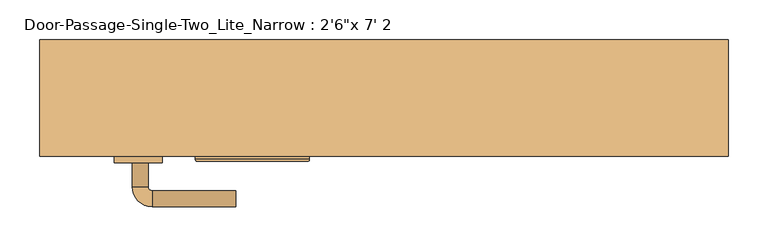
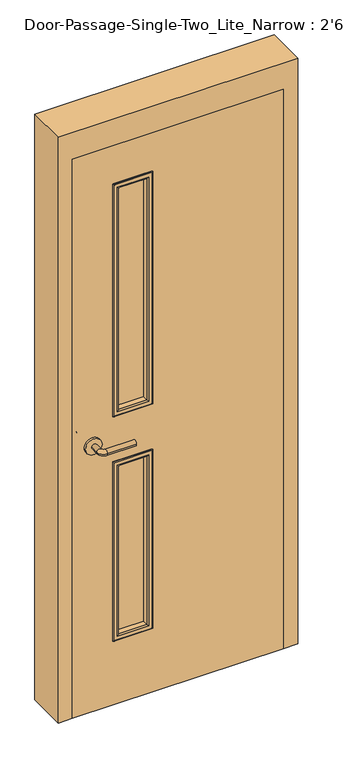
"""IFC4 building model written with IfcOpenShell, lengths in millimetres: door geometry."""

from ifc_helpers import new_model, si_unit, point, frame, frame_2d, origin, place, context, project, spatial, polyline, circle_curve, ellipse_curve, trimmed, segment, composite_curve, outline, extrude, faceted_brep, source, transform, mapped, element, save
from ifc_brep_helpers import plane_surface, cylinder_surface, revolved_surface, advanced_brep


def door_bcd1f9a3(model_context):
    return source(origin(), model_context, "Body", "SolidModel", [
        advanced_brep(
        [(-315.990625, 14.35, 1016.0), (-295.990625, 14.35, 1016.0), (-315.990625, 44.35, 1016.0), (-295.990625, 44.35, 1016.0), (-290.990625, 49.35, 1016.0), (-290.990625, 69.35, 1016.0), (-185.990625, 69.35, 1016.0), (-185.990625, 49.35, 1016.0)],
        [
            (0, 1, circle_curve(frame((-305.990625, 14.35, 1016.0), z_axis=(0.0, -1.0, 0.0), x_axis=(1.0, 0.0, 0.0)), 10.0)),
            (1, 0, circle_curve(frame((-305.990625, 14.35, 1016.0), z_axis=(0.0, -1.0, 0.0), x_axis=(1.0, 0.0, 0.0)), 10.0)),
            (0, 2),
            (2, 3, circle_curve(frame((-305.990625, 44.35, 1016.0), z_axis=(0.0, -1.0, 0.0), x_axis=(1.0, 0.0, 0.0)), 10.0)),
            (3, 1),
            (3, 2, circle_curve(frame((-305.990625, 44.35, 1016.0), z_axis=(0.0, -1.0, 0.0), x_axis=(1.0, 0.0, 0.0)), 10.0)),
            (4, 3, circle_curve(frame((-290.990625, 44.35, 1016.0), z_axis=(0.0, 0.0, 1.0), x_axis=(-1.0, 0.0, 0.0)), 5.0)),
            (2, 5, circle_curve(frame((-290.990625, 44.35, 1016.0), z_axis=(0.0, 0.0, -1.0), x_axis=(-1.0, 0.0, 0.0)), 25.0)),
            (5, 4, circle_curve(frame((-290.990625, 59.35, 1016.0), z_axis=(-1.0, 0.0, 0.0), x_axis=(0.0, -1.0, 0.0)), 10.0)),
            (4, 5, circle_curve(frame((-290.990625, 59.35, 1016.0), z_axis=(-1.0, 0.0, 0.0), x_axis=(0.0, -1.0, 0.0)), 10.0)),
            (6, 7, circle_curve(frame((-185.990625, 59.35, 1016.0), z_axis=(1.0, 0.0, 0.0), x_axis=(0.0, -1.0, 0.0)), 10.0)),
            (7, 6, circle_curve(frame((-185.990625, 59.35, 1016.0), z_axis=(1.0, 0.0, 0.0), x_axis=(0.0, -1.0, 0.0)), 10.0)),
            (5, 6),
            (7, 4),
        ],
        [
            plane_surface(frame((-305.990625, 14.35, 1016.0), z_axis=(0.0, -1.0, 0.0), x_axis=(0.0, 0.0, 1.0))),
            cylinder_surface(frame((-305.990625, 14.35, 1016.0), z_axis=(0.0, -1.0, 0.0), x_axis=(1.0, 0.0, 0.0)), 10.0),
            revolved_surface(trimmed(ellipse_curve(frame((-305.990625, 44.35, 1016.0), z_axis=(0.0, -1.0, 0.0), x_axis=(1.0, 0.0, 0.0)), 10.0, 10.0), [point((-315.990625, 44.35, 1016.0))], [point((-295.990625, 44.35, 1016.0))], True, "CARTESIAN"), (-290.990625, 44.35, 1016.0), (0.0, 0.0, -1.0)),
            revolved_surface(trimmed(ellipse_curve(frame((-305.990625, 44.35, 1016.0), z_axis=(0.0, -1.0, 0.0), x_axis=(1.0, 0.0, 0.0)), 10.0, 10.0), [point((-295.990625, 44.35, 1016.0))], [point((-315.990625, 44.35, 1016.0))], True, "CARTESIAN"), (-290.990625, 44.35, 1016.0), (0.0, 0.0, -1.0)),
            plane_surface(frame((-185.990625, 59.35, 1016.0), z_axis=(1.0, 0.0, 0.0), x_axis=(0.0, 0.0, 1.0))),
            cylinder_surface(frame((-290.990625, 59.35, 1016.0), z_axis=(-1.0, 0.0, 0.0), x_axis=(0.0, -1.0, 0.0)), 10.0),
        ],
        [
            (0, [[1, 2]]),
            (1, [[-1, 3, 4, 5]]),
            (1, [[-2, -5, 6, -3]]),
            (2, [[7, -4, 8, 9]]),
            (3, [[-8, -6, -7, 10]]),
            (4, [[11, 12]]),
            (5, [[-9, 13, -12, 14]]),
            (5, [[-10, -14, -11, -13]]),
        ],
    ),
        extrude(outline(composite_curve([segment(trimmed(circle_curve(frame_2d((1016.0, -308.490625)), 30.0), [point((1016.0, -338.490625))], [point((1016.0, -278.490625))], False, "CARTESIAN"), True, "CONTINUOUS"), segment(trimmed(circle_curve(frame_2d((1016.0, -308.490625)), 30.0), [point((1016.0, -278.490625))], [point((1016.0, -338.490625))], False, "CARTESIAN"), True, "CONTINUOUS")], self_intersect=False)), frame((0.0, 6.35, 0.0), z_axis=(0.0, 1.0, 0.0), x_axis=(0.0, 0.0, 1.0)), (0.0, 0.0, 1.0), 8.0),
        advanced_brep(
        [(-315.990625, -46.1, 1016.0), (-295.990625, -46.1, 1016.0), (-295.990625, -76.1, 1016.0), (-315.990625, -76.1, 1016.0), (-290.990625, -81.1, 1016.0), (-290.990625, -101.1, 1016.0), (-185.990625, -101.1, 1016.0), (-185.990625, -81.1, 1016.0)],
        [
            (0, 1, circle_curve(frame((-305.990625, -46.1, 1016.0), z_axis=(0.0, 1.0, 0.0), x_axis=(1.0, 0.0, 0.0)), 10.0)),
            (1, 0, circle_curve(frame((-305.990625, -46.1, 1016.0), z_axis=(0.0, 1.0, 0.0), x_axis=(1.0, 0.0, 0.0)), 10.0)),
            (1, 2),
            (2, 3, circle_curve(frame((-305.990625, -76.1, 1016.0), z_axis=(0.0, 1.0, 0.0), x_axis=(1.0, 0.0, 0.0)), 10.0)),
            (3, 0),
            (3, 2, circle_curve(frame((-305.990625, -76.1, 1016.0), z_axis=(0.0, 1.0, 0.0), x_axis=(1.0, 0.0, 0.0)), 10.0)),
            (4, 5, circle_curve(frame((-290.990625, -91.1, 1016.0), z_axis=(-1.0, 0.0, 0.0), x_axis=(0.0, 1.0, 0.0)), 10.0)),
            (5, 3, circle_curve(frame((-290.990625, -76.1, 1016.0), z_axis=(0.0, 0.0, -1.0), x_axis=(-1.0, 0.0, 0.0)), 25.0)),
            (2, 4, circle_curve(frame((-290.990625, -76.1, 1016.0), z_axis=(0.0, 0.0, 1.0), x_axis=(-1.0, 0.0, 0.0)), 5.0)),
            (5, 4, circle_curve(frame((-290.990625, -91.1, 1016.0), z_axis=(-1.0, 0.0, 0.0), x_axis=(0.0, 1.0, 0.0)), 10.0)),
            (6, 7, circle_curve(frame((-185.990625, -91.1, 1016.0), z_axis=(1.0, 0.0, 0.0), x_axis=(0.0, 1.0, 0.0)), 10.0)),
            (7, 6, circle_curve(frame((-185.990625, -91.1, 1016.0), z_axis=(1.0, 0.0, 0.0), x_axis=(0.0, 1.0, 0.0)), 10.0)),
            (4, 7),
            (6, 5),
        ],
        [
            plane_surface(frame((-305.990625, -46.1, 1016.0), z_axis=(0.0, 1.0, 0.0), x_axis=(0.0, 0.0, 1.0))),
            cylinder_surface(frame((-305.990625, -46.1, 1016.0), z_axis=(0.0, 1.0, 0.0), x_axis=(1.0, 0.0, 0.0)), 10.0),
            revolved_surface(trimmed(ellipse_curve(frame((-305.990625, -76.1, 1016.0), z_axis=(0.0, -1.0, 0.0), x_axis=(1.0, 0.0, 0.0)), 10.0, 10.0), [point((-315.990625, -76.1, 1016.0))], [point((-295.990625, -76.1, 1016.0))], True, "CARTESIAN"), (-290.990625, -76.1, 1016.0), (0.0, 0.0, -1.0)),
            revolved_surface(trimmed(ellipse_curve(frame((-305.990625, -76.1, 1016.0), z_axis=(0.0, -1.0, 0.0), x_axis=(1.0, 0.0, 0.0)), 10.0, 10.0), [point((-295.990625, -76.1, 1016.0))], [point((-315.990625, -76.1, 1016.0))], True, "CARTESIAN"), (-290.990625, -76.1, 1016.0), (0.0, 0.0, -1.0)),
            plane_surface(frame((-185.990625, -91.1, 1016.0), z_axis=(1.0, 0.0, 0.0), x_axis=(0.0, 0.0, 1.0))),
            cylinder_surface(frame((-290.990625, -91.1, 1016.0), z_axis=(-1.0, 0.0, 0.0), x_axis=(0.0, 1.0, 0.0)), 10.0),
        ],
        [
            (0, [[1, 2]]),
            (1, [[3, 4, 5, -2]]),
            (1, [[-5, 6, -3, -1]]),
            (2, [[7, 8, -4, 9]]),
            (3, [[10, -9, -6, -8]]),
            (4, [[11, 12]]),
            (5, [[13, -11, 14, -7]]),
            (5, [[-14, -12, -13, -10]]),
        ],
    ),
        extrude(outline(composite_curve([segment(trimmed(circle_curve(frame_2d((1016.0, -308.490625)), 30.0), [point((1016.0, -338.490625))], [point((1016.0, -278.490625))], False, "CARTESIAN"), True, "CONTINUOUS"), segment(trimmed(circle_curve(frame_2d((1016.0, -308.490625)), 30.0), [point((1016.0, -278.490625))], [point((1016.0, -338.490625))], False, "CARTESIAN"), True, "CONTINUOUS")], self_intersect=False)), frame((0.0, -46.1, 0.0), z_axis=(0.0, 1.0, 0.0), x_axis=(0.0, 0.0, 1.0)), (0.0, 0.0, 1.0), 8.0),
        extrude(outline(polyline([(2133.6, -381.0), (0.0, -381.0), (0.0, 381.0), (2133.6, 381.0), (2133.6, -381.0)]), holes=[polyline([(1981.2, -228.6), (1981.2, -101.6), (1111.25, -101.6), (1111.25, -228.6), (1981.2, -228.6)]), polyline([(920.75, -228.6), (920.75, -101.6), (254.0, -101.6), (254.0, -228.6), (920.75, -228.6)])]), frame((0.0, -38.1, 0.0), z_axis=(0.0, 1.0, 0.0), x_axis=(0.0, 0.0, 1.0)), (0.0, 0.0, 1.0), 44.45),
        faceted_brep([(381.0, 11.1125, 0.0), (365.125, 11.1125, 0.0), (365.125, 58.7375, 0.0), (381.0, 58.7375, 0.0), (381.0, 107.95, 0.0), (431.8, 107.95, 0.0), (431.8, -38.1, 0.0), (381.0, -38.1, 0.0), (381.0, -38.1, 2133.6), (381.0, 11.1125, 2133.6), (431.8, -38.1, 2235.2), (-431.8, -38.1, 2235.2), (-431.8, -38.1, 0.0), (-381.0, -38.1, 0.0), (-381.0, -38.1, 2133.6), (431.8, 107.95, 2235.2), (381.0, 107.95, 2133.6), (-381.0, 107.95, 2133.6), (-381.0, 107.95, 0.0), (-431.8, 107.95, 0.0), (-431.8, 107.95, 2235.2), (381.0, 58.7375, 2133.6), (365.125, 58.7375, 2117.725), (-365.125, 58.7375, 2117.725), (-365.125, 58.7375, 0.0), (-381.0, 58.7375, 0.0), (-381.0, 58.7375, 2133.6), (365.125, 11.1125, 2117.725), (-381.0, 11.1125, 2133.6), (-381.0, 11.1125, 0.0), (-365.125, 11.1125, 0.0), (-365.125, 11.1125, 2117.725)], [[[0, 1, 2, 3, 4, 5, 6, 7]], [[7, 8, 9, 0]], [[6, 10, 11, 12, 13, 14, 8, 7]], [[5, 15, 10, 6]], [[4, 16, 17, 18, 19, 20, 15, 5]], [[3, 21, 16, 4]], [[2, 22, 23, 24, 25, 26, 21, 3]], [[1, 27, 22, 2]], [[0, 9, 28, 29, 30, 31, 27, 1]], [[8, 14, 28, 9]], [[16, 21, 26, 17]], [[22, 27, 31, 23]], [[12, 19, 18, 25, 24, 30, 29, 13]], [[13, 29, 28, 14]], [[11, 20, 19, 12]], [[17, 26, 25, 18]], [[23, 31, 30, 24]], [[15, 20, 11, 10]]]),
        extrude(outline(polyline([(-101.6, -12.7), (-101.6, -19.05), (-228.6, -19.05), (-228.6, -12.7), (-101.6, -12.7)])), frame((0.0, 0.0, 1111.25), z_axis=(0.0, 0.0, 1.0), x_axis=(1.0, 0.0, 0.0)), (0.0, 0.0, 1.0), 869.95),
        extrude(outline(polyline([(-101.6, -12.7), (-101.6, -19.05), (-228.6, -19.05), (-228.6, -12.7), (-101.6, -12.7)])), frame((0.0, 0.0, 254.0), z_axis=(0.0, 0.0, 1.0), x_axis=(1.0, 0.0, 0.0)), (0.0, 0.0, 1.0), 666.75),
        advanced_brep(
        [(-228.6, -19.05, 1981.2), (-228.6, -19.05, 1111.25), (-228.6, -38.1, 1111.25), (-228.6, -38.1, 1981.2), (-216.6, -39.1, 1969.2), (-216.6, -39.1, 1123.25), (-216.6, -19.05, 1123.25), (-216.6, -19.05, 1969.2), (-221.6, -44.1, 1974.2), (-221.6, -44.1, 1118.25), (-236.6, -42.1, 1989.2), (-236.6, -42.1, 1103.25), (-234.6, -44.1, 1105.25), (-234.6, -44.1, 1987.2), (-236.6, -38.1, 1989.2), (-236.6, -38.1, 1103.25), (-101.6, -19.05, 1111.25), (-101.6, -38.1, 1111.25), (-113.6, -39.1, 1123.25), (-113.6, -19.05, 1123.25), (-108.6, -44.1, 1118.25), (-93.6, -42.1, 1103.25), (-95.6, -44.1, 1105.25), (-93.6, -38.1, 1103.25), (-101.6, -19.05, 1981.2), (-101.6, -38.1, 1981.2), (-113.6, -39.1, 1969.2), (-113.6, -19.05, 1969.2), (-108.6, -44.1, 1974.2), (-93.6, -42.1, 1989.2), (-95.6, -44.1, 1987.2), (-93.6, -38.1, 1989.2)],
        [
            (0, 1),
            (1, 2),
            (2, 3),
            (3, 0),
            (4, 5),
            (5, 6),
            (6, 7),
            (7, 4),
            (8, 9),
            (9, 5, ellipse_curve(frame((-221.6, -39.1, 1118.25), z_axis=(-0.7071067811865475, 0.0, 0.7071067811865475), x_axis=(0.7071067811865474, 0.0, 0.7071067811865476)), 7.0710678, 5.0)),
            (4, 8, ellipse_curve(frame((-221.6, -39.1, 1974.2), z_axis=(-0.7071067811865475, 0.0, -0.7071067811865475), x_axis=(-0.7071067811865474, 0.0, 0.7071067811865476)), 7.0710678, 5.0)),
            (10, 11),
            (11, 12, ellipse_curve(frame((-234.6, -42.1, 1105.25), z_axis=(-0.7071067811865475, 0.0, 0.7071067811865475), x_axis=(0.7071067811865474, 0.0, 0.7071067811865476)), 2.8284271, 2.0)),
            (12, 13),
            (13, 10, ellipse_curve(frame((-234.6, -42.1, 1987.2), z_axis=(-0.7071067811865475, 0.0, -0.7071067811865475), x_axis=(-0.7071067811865474, 0.0, 0.7071067811865476)), 2.8284271, 2.0)),
            (14, 15),
            (15, 11),
            (10, 14),
            (1, 16),
            (16, 17),
            (17, 2),
            (5, 18),
            (18, 19),
            (19, 6),
            (9, 20),
            (20, 18, ellipse_curve(frame((-108.6, -39.1, 1118.25), z_axis=(-0.7071067811865475, 0.0, -0.7071067811865475), x_axis=(-0.7071067811865476, 0.0, 0.7071067811865474)), 7.0710678, 5.0)),
            (11, 21),
            (21, 22, ellipse_curve(frame((-95.6, -42.1, 1105.25), z_axis=(-0.7071067811865475, 0.0, -0.7071067811865475), x_axis=(-0.7071067811865476, 0.0, 0.7071067811865474)), 2.8284271, 2.0)),
            (22, 12),
            (15, 23),
            (23, 21),
            (16, 24),
            (24, 25),
            (25, 17),
            (18, 26),
            (26, 27),
            (27, 19),
            (20, 28),
            (28, 26, ellipse_curve(frame((-108.6, -39.1, 1974.2), z_axis=(0.7071067811865475, 0.0, -0.7071067811865475), x_axis=(-0.7071067811865474, 0.0, -0.7071067811865476)), 7.0710678, 5.0)),
            (21, 29),
            (29, 30, ellipse_curve(frame((-95.6, -42.1, 1987.2), z_axis=(0.7071067811865475, 0.0, -0.7071067811865475), x_axis=(-0.7071067811865474, 0.0, -0.7071067811865476)), 2.8284271, 2.0)),
            (30, 22),
            (23, 31),
            (31, 29),
            (14, 31),
            (25, 3),
            (24, 0),
            (27, 7),
            (26, 4),
            (28, 8),
            (30, 13),
            (29, 10),
        ],
        [
            plane_surface(frame((-228.6, -38.1, 1981.2), z_axis=(-1.0, 0.0, 0.0), x_axis=(0.0, 0.0, -1.0))),
            plane_surface(frame((-216.6, -19.05, 1969.2), z_axis=(1.0, 0.0, 0.0), x_axis=(0.0, 0.0, -1.0))),
            cylinder_surface(frame((-221.6, -39.1, 1981.2), z_axis=(0.0, 0.0, 1.0), x_axis=(-1.0, 0.0, 0.0)), 5.0),
            cylinder_surface(frame((-234.6, -42.1, 1981.2), z_axis=(0.0, 0.0, 1.0), x_axis=(-1.0, 0.0, 0.0)), 2.0),
            plane_surface(frame((-236.6, -42.1, 1989.2), z_axis=(-1.0, 0.0, 0.0), x_axis=(0.0, 0.0, -1.0))),
            plane_surface(frame((-228.6, -38.1, 1111.25), z_axis=(0.0, 0.0, -1.0), x_axis=(1.0, 0.0, 0.0))),
            plane_surface(frame((-216.6, -19.05, 1123.25), z_axis=(0.0, 0.0, 1.0), x_axis=(1.0, 0.0, 0.0))),
            cylinder_surface(frame((-228.6, -39.1, 1118.25), z_axis=(-1.0, 0.0, 0.0), x_axis=(0.0, 0.0, -1.0)), 5.0),
            cylinder_surface(frame((-228.6, -42.1, 1105.25), z_axis=(-1.0, 0.0, 0.0), x_axis=(0.0, 0.0, -1.0)), 2.0),
            plane_surface(frame((-236.6, -42.1, 1103.25), z_axis=(0.0, 0.0, -1.0), x_axis=(1.0, 0.0, 0.0))),
            plane_surface(frame((-101.6, -38.1, 1111.25), z_axis=(1.0, 0.0, 0.0), x_axis=(0.0, 0.0, 1.0))),
            plane_surface(frame((-113.6, -19.05, 1123.25), z_axis=(-1.0, 0.0, 0.0), x_axis=(0.0, 0.0, 1.0))),
            cylinder_surface(frame((-108.6, -39.1, 1111.25), z_axis=(0.0, 0.0, -1.0), x_axis=(1.0, 0.0, 0.0)), 5.0),
            cylinder_surface(frame((-95.6, -42.1, 1111.25), z_axis=(0.0, 0.0, -1.0), x_axis=(1.0, 0.0, 0.0)), 2.0),
            plane_surface(frame((-93.6, -42.1, 1103.25), z_axis=(1.0, 0.0, 0.0), x_axis=(0.0, 0.0, 1.0))),
            plane_surface(frame((-93.6, -38.1, 1989.2), z_axis=(0.0, 1.0, 0.0), x_axis=(-1.0, 0.0, 0.0))),
            plane_surface(frame((-101.6, -38.1, 1981.2), z_axis=(0.0, 0.0, 1.0), x_axis=(-1.0, 0.0, 0.0))),
            plane_surface(frame((-101.6, -19.05, 1981.2), z_axis=(0.0, 1.0, 0.0), x_axis=(-1.0, 0.0, 0.0))),
            plane_surface(frame((-113.6, -19.05, 1969.2), z_axis=(0.0, 0.0, -1.0), x_axis=(-1.0, 0.0, 0.0))),
            cylinder_surface(frame((-101.6, -39.1, 1974.2), z_axis=(1.0, 0.0, 0.0), x_axis=(0.0, 0.0, 1.0)), 5.0),
            plane_surface(frame((-108.6, -44.1, 1974.2), z_axis=(0.0, -1.0, 0.0), x_axis=(-1.0, 0.0, 0.0))),
            cylinder_surface(frame((-101.6, -42.1, 1987.2), z_axis=(1.0, 0.0, 0.0), x_axis=(0.0, 0.0, 1.0)), 2.0),
            plane_surface(frame((-93.6, -42.1, 1989.2), z_axis=(0.0, 0.0, 1.0), x_axis=(-1.0, 0.0, 0.0))),
        ],
        [
            (0, [[1, 2, 3, 4]]),
            (1, [[5, 6, 7, 8]]),
            (2, [[9, 10, -5, 11]]),
            (3, [[12, 13, 14, 15]]),
            (4, [[16, 17, -12, 18]]),
            (5, [[19, 20, 21, -2]]),
            (6, [[22, 23, 24, -6]]),
            (7, [[25, 26, -22, -10]]),
            (8, [[27, 28, 29, -13]]),
            (9, [[30, 31, -27, -17]]),
            (10, [[32, 33, 34, -20]]),
            (11, [[35, 36, 37, -23]]),
            (12, [[38, 39, -35, -26]]),
            (13, [[40, 41, 42, -28]]),
            (14, [[43, 44, -40, -31]]),
            (15, [[-16, 45, -43, -30], [-3, -21, -34, 46]]),
            (16, [[47, -4, -46, -33]]),
            (17, [[-1, -47, -32, -19], [-7, -24, -37, 48]]),
            (18, [[49, -8, -48, -36]]),
            (19, [[50, -11, -49, -39]]),
            (20, [[-14, -29, -42, 51], [-9, -50, -38, -25]]),
            (21, [[52, -15, -51, -41]]),
            (22, [[-45, -18, -52, -44]]),
        ],
    ),
        advanced_brep(
        [(-228.6, -12.7, 1111.25), (-228.6, -12.7, 1981.2), (-228.6, 6.35, 1981.2), (-228.6, 6.35, 1111.25), (-216.6, 7.35, 1123.25), (-216.6, 7.35, 1969.2), (-216.6, -12.7, 1969.2), (-216.6, -12.7, 1123.25), (-221.6, 12.35, 1118.25), (-221.6, 12.35, 1974.2), (-236.6, 10.35, 1103.25), (-236.6, 10.35, 1989.2), (-234.6, 12.35, 1987.2), (-234.6, 12.35, 1105.25), (-236.6, 6.35, 1103.25), (-236.6, 6.35, 1989.2), (-101.6, -12.7, 1981.2), (-101.6, 6.35, 1981.2), (-113.6, 7.35, 1969.2), (-113.6, -12.7, 1969.2), (-108.6, 12.35, 1974.2), (-93.6, 10.35, 1989.2), (-95.6, 12.35, 1987.2), (-93.6, 6.35, 1989.2), (-101.6, -12.7, 1111.25), (-101.6, 6.35, 1111.25), (-113.6, 7.35, 1123.25), (-113.6, -12.7, 1123.25), (-108.6, 12.35, 1118.25), (-93.6, 10.35, 1103.25), (-95.6, 12.35, 1105.25), (-93.6, 6.35, 1103.25)],
        [
            (0, 1),
            (1, 2),
            (2, 3),
            (3, 0),
            (4, 5),
            (5, 6),
            (6, 7),
            (7, 4),
            (8, 9),
            (9, 5, ellipse_curve(frame((-221.6, 7.35, 1974.2), z_axis=(-0.7071067811865475, 0.0, -0.7071067811865475), x_axis=(0.7071067811865474, 0.0, -0.7071067811865476)), 7.0710678, 5.0)),
            (4, 8, ellipse_curve(frame((-221.6, 7.35, 1118.25), z_axis=(-0.7071067811865475, 0.0, 0.7071067811865475), x_axis=(-0.7071067811865474, 0.0, -0.7071067811865476)), 7.0710678, 5.0)),
            (10, 11),
            (11, 12, ellipse_curve(frame((-234.6, 10.35, 1987.2), z_axis=(-0.7071067811865475, 0.0, -0.7071067811865475), x_axis=(0.7071067811865474, 0.0, -0.7071067811865476)), 2.8284271, 2.0)),
            (12, 13),
            (13, 10, ellipse_curve(frame((-234.6, 10.35, 1105.25), z_axis=(-0.7071067811865475, 0.0, 0.7071067811865475), x_axis=(-0.7071067811865474, 0.0, -0.7071067811865476)), 2.8284271, 2.0)),
            (14, 15),
            (15, 11),
            (10, 14),
            (1, 16),
            (16, 17),
            (17, 2),
            (5, 18),
            (18, 19),
            (19, 6),
            (9, 20),
            (20, 18, ellipse_curve(frame((-108.6, 7.35, 1974.2), z_axis=(-0.7071067811865475, 0.0, 0.7071067811865475), x_axis=(-0.7071067811865476, 0.0, -0.7071067811865474)), 7.0710678, 5.0)),
            (11, 21),
            (21, 22, ellipse_curve(frame((-95.6, 10.35, 1987.2), z_axis=(-0.7071067811865475, 0.0, 0.7071067811865475), x_axis=(-0.7071067811865476, 0.0, -0.7071067811865474)), 2.8284271, 2.0)),
            (22, 12),
            (15, 23),
            (23, 21),
            (16, 24),
            (24, 25),
            (25, 17),
            (18, 26),
            (26, 27),
            (27, 19),
            (20, 28),
            (28, 26, ellipse_curve(frame((-108.6, 7.35, 1118.25), z_axis=(0.7071067811865475, 0.0, 0.7071067811865475), x_axis=(-0.7071067811865474, 0.0, 0.7071067811865476)), 7.0710678, 5.0)),
            (21, 29),
            (29, 30, ellipse_curve(frame((-95.6, 10.35, 1105.25), z_axis=(0.7071067811865475, 0.0, 0.7071067811865475), x_axis=(-0.7071067811865474, 0.0, 0.7071067811865476)), 2.8284271, 2.0)),
            (30, 22),
            (23, 31),
            (31, 29),
            (14, 31),
            (25, 3),
            (24, 0),
            (27, 7),
            (26, 4),
            (28, 8),
            (30, 13),
            (29, 10),
        ],
        [
            plane_surface(frame((-228.6, 6.35, 1111.25), z_axis=(-1.0, 0.0, 0.0), x_axis=(0.0, 0.0, 1.0))),
            plane_surface(frame((-216.6, -12.7, 1123.25), z_axis=(1.0, 0.0, 0.0), x_axis=(0.0, 0.0, 1.0))),
            cylinder_surface(frame((-221.6, 7.35, 1111.25), z_axis=(0.0, 0.0, -1.0), x_axis=(-1.0, 0.0, 0.0)), 5.0),
            cylinder_surface(frame((-234.6, 10.35, 1111.25), z_axis=(0.0, 0.0, -1.0), x_axis=(-1.0, 0.0, 0.0)), 2.0),
            plane_surface(frame((-236.6, 10.35, 1103.25), z_axis=(-1.0, 0.0, 0.0), x_axis=(0.0, 0.0, 1.0))),
            plane_surface(frame((-228.6, 6.35, 1981.2), z_axis=(0.0, 0.0, 1.0), x_axis=(1.0, 0.0, 0.0))),
            plane_surface(frame((-216.6, -12.7, 1969.2), z_axis=(0.0, 0.0, -1.0), x_axis=(1.0, 0.0, 0.0))),
            cylinder_surface(frame((-228.6, 7.35, 1974.2), z_axis=(-1.0, 0.0, 0.0), x_axis=(0.0, 0.0, 1.0)), 5.0),
            cylinder_surface(frame((-228.6, 10.35, 1987.2), z_axis=(-1.0, 0.0, 0.0), x_axis=(0.0, 0.0, 1.0)), 2.0),
            plane_surface(frame((-236.6, 10.35, 1989.2), z_axis=(0.0, 0.0, 1.0), x_axis=(1.0, 0.0, 0.0))),
            plane_surface(frame((-101.6, 6.35, 1981.2), z_axis=(1.0, 0.0, 0.0), x_axis=(0.0, 0.0, -1.0))),
            plane_surface(frame((-113.6, -12.7, 1969.2), z_axis=(-1.0, 0.0, 0.0), x_axis=(0.0, 0.0, -1.0))),
            cylinder_surface(frame((-108.6, 7.35, 1981.2), z_axis=(0.0, 0.0, 1.0), x_axis=(1.0, 0.0, 0.0)), 5.0),
            cylinder_surface(frame((-95.6, 10.35, 1981.2), z_axis=(0.0, 0.0, 1.0), x_axis=(1.0, 0.0, 0.0)), 2.0),
            plane_surface(frame((-93.6, 10.35, 1989.2), z_axis=(1.0, 0.0, 0.0), x_axis=(0.0, 0.0, -1.0))),
            plane_surface(frame((-93.6, 6.35, 1103.25), z_axis=(0.0, -1.0, 0.0), x_axis=(-1.0, 0.0, 0.0))),
            plane_surface(frame((-101.6, 6.35, 1111.25), z_axis=(0.0, 0.0, -1.0), x_axis=(-1.0, 0.0, 0.0))),
            plane_surface(frame((-101.6, -12.7, 1111.25), z_axis=(0.0, -1.0, 0.0), x_axis=(-1.0, 0.0, 0.0))),
            plane_surface(frame((-113.6, -12.7, 1123.25), z_axis=(0.0, 0.0, 1.0), x_axis=(-1.0, 0.0, 0.0))),
            cylinder_surface(frame((-101.6, 7.35, 1118.25), z_axis=(1.0, 0.0, 0.0), x_axis=(0.0, 0.0, -1.0)), 5.0),
            plane_surface(frame((-108.6, 12.35, 1118.25), z_axis=(0.0, 1.0, 0.0), x_axis=(-1.0, 0.0, 0.0))),
            cylinder_surface(frame((-101.6, 10.35, 1105.25), z_axis=(1.0, 0.0, 0.0), x_axis=(0.0, 0.0, -1.0)), 2.0),
            plane_surface(frame((-93.6, 10.35, 1103.25), z_axis=(0.0, 0.0, -1.0), x_axis=(-1.0, 0.0, 0.0))),
        ],
        [
            (0, [[1, 2, 3, 4]]),
            (1, [[5, 6, 7, 8]]),
            (2, [[9, 10, -5, 11]]),
            (3, [[12, 13, 14, 15]]),
            (4, [[16, 17, -12, 18]]),
            (5, [[19, 20, 21, -2]]),
            (6, [[22, 23, 24, -6]]),
            (7, [[25, 26, -22, -10]]),
            (8, [[27, 28, 29, -13]]),
            (9, [[30, 31, -27, -17]]),
            (10, [[32, 33, 34, -20]]),
            (11, [[35, 36, 37, -23]]),
            (12, [[38, 39, -35, -26]]),
            (13, [[40, 41, 42, -28]]),
            (14, [[43, 44, -40, -31]]),
            (15, [[-16, 45, -43, -30], [-3, -21, -34, 46]]),
            (16, [[47, -4, -46, -33]]),
            (17, [[-1, -47, -32, -19], [-7, -24, -37, 48]]),
            (18, [[49, -8, -48, -36]]),
            (19, [[50, -11, -49, -39]]),
            (20, [[-14, -29, -42, 51], [-9, -50, -38, -25]]),
            (21, [[52, -15, -51, -41]]),
            (22, [[-45, -18, -52, -44]]),
        ],
    ),
        advanced_brep(
        [(-228.6, -19.05, 920.75), (-228.6, -19.05, 254.0), (-228.6, -38.1, 254.0), (-228.6, -38.1, 920.75), (-216.6, -39.1, 908.75), (-216.6, -39.1, 266.0), (-216.6, -19.05, 266.0), (-216.6, -19.05, 908.75), (-221.6, -44.1, 913.75), (-221.6, -44.1, 261.0), (-236.6, -42.1, 928.75), (-236.6, -42.1, 246.0), (-234.6, -44.1, 248.0), (-234.6, -44.1, 926.75), (-236.6, -38.1, 928.75), (-236.6, -38.1, 246.0), (-101.6, -19.05, 254.0), (-101.6, -38.1, 254.0), (-113.6, -39.1, 266.0), (-113.6, -19.05, 266.0), (-108.6, -44.1, 261.0), (-93.6, -42.1, 246.0), (-95.6, -44.1, 248.0), (-93.6, -38.1, 246.0), (-101.6, -19.05, 920.75), (-101.6, -38.1, 920.75), (-113.6, -39.1, 908.75), (-113.6, -19.05, 908.75), (-108.6, -44.1, 913.75), (-93.6, -42.1, 928.75), (-95.6, -44.1, 926.75), (-93.6, -38.1, 928.75)],
        [
            (0, 1),
            (1, 2),
            (2, 3),
            (3, 0),
            (4, 5),
            (5, 6),
            (6, 7),
            (7, 4),
            (8, 9),
            (9, 5, ellipse_curve(frame((-221.6, -39.1, 261.0), z_axis=(-0.7071067811865475, 0.0, 0.7071067811865475), x_axis=(0.7071067811865474, 0.0, 0.7071067811865476)), 7.0710678, 5.0)),
            (4, 8, ellipse_curve(frame((-221.6, -39.1, 913.75), z_axis=(-0.7071067811865475, 0.0, -0.7071067811865475), x_axis=(-0.7071067811865474, 0.0, 0.7071067811865476)), 7.0710678, 5.0)),
            (10, 11),
            (11, 12, ellipse_curve(frame((-234.6, -42.1, 248.0), z_axis=(-0.7071067811865475, 0.0, 0.7071067811865475), x_axis=(0.7071067811865474, 0.0, 0.7071067811865476)), 2.8284271, 2.0)),
            (12, 13),
            (13, 10, ellipse_curve(frame((-234.6, -42.1, 926.75), z_axis=(-0.7071067811865475, 0.0, -0.7071067811865475), x_axis=(-0.7071067811865474, 0.0, 0.7071067811865476)), 2.8284271, 2.0)),
            (14, 15),
            (15, 11),
            (10, 14),
            (1, 16),
            (16, 17),
            (17, 2),
            (5, 18),
            (18, 19),
            (19, 6),
            (9, 20),
            (20, 18, ellipse_curve(frame((-108.6, -39.1, 261.0), z_axis=(-0.7071067811865475, 0.0, -0.7071067811865475), x_axis=(-0.7071067811865476, 0.0, 0.7071067811865474)), 7.0710678, 5.0)),
            (11, 21),
            (21, 22, ellipse_curve(frame((-95.6, -42.1, 248.0), z_axis=(-0.7071067811865475, 0.0, -0.7071067811865475), x_axis=(-0.7071067811865476, 0.0, 0.7071067811865474)), 2.8284271, 2.0)),
            (22, 12),
            (15, 23),
            (23, 21),
            (16, 24),
            (24, 25),
            (25, 17),
            (18, 26),
            (26, 27),
            (27, 19),
            (20, 28),
            (28, 26, ellipse_curve(frame((-108.6, -39.1, 913.75), z_axis=(0.7071067811865475, 0.0, -0.7071067811865475), x_axis=(-0.7071067811865474, 0.0, -0.7071067811865476)), 7.0710678, 5.0)),
            (21, 29),
            (29, 30, ellipse_curve(frame((-95.6, -42.1, 926.75), z_axis=(0.7071067811865475, 0.0, -0.7071067811865475), x_axis=(-0.7071067811865474, 0.0, -0.7071067811865476)), 2.8284271, 2.0)),
            (30, 22),
            (23, 31),
            (31, 29),
            (14, 31),
            (25, 3),
            (24, 0),
            (27, 7),
            (26, 4),
            (28, 8),
            (30, 13),
            (29, 10),
        ],
        [
            plane_surface(frame((-228.6, -38.1, 920.75), z_axis=(-1.0, 0.0, 0.0), x_axis=(0.0, 0.0, -1.0))),
            plane_surface(frame((-216.6, -19.05, 908.75), z_axis=(1.0, 0.0, 0.0), x_axis=(0.0, 0.0, -1.0))),
            cylinder_surface(frame((-221.6, -39.1, 920.75), z_axis=(0.0, 0.0, 1.0), x_axis=(-1.0, 0.0, 0.0)), 5.0),
            cylinder_surface(frame((-234.6, -42.1, 920.75), z_axis=(0.0, 0.0, 1.0), x_axis=(-1.0, 0.0, 0.0)), 2.0),
            plane_surface(frame((-236.6, -42.1, 928.75), z_axis=(-1.0, 0.0, 0.0), x_axis=(0.0, 0.0, -1.0))),
            plane_surface(frame((-228.6, -38.1, 254.0), z_axis=(0.0, 0.0, -1.0), x_axis=(1.0, 0.0, 0.0))),
            plane_surface(frame((-216.6, -19.05, 266.0), z_axis=(0.0, 0.0, 1.0), x_axis=(1.0, 0.0, 0.0))),
            cylinder_surface(frame((-228.6, -39.1, 261.0), z_axis=(-1.0, 0.0, 0.0), x_axis=(0.0, 0.0, -1.0)), 5.0),
            cylinder_surface(frame((-228.6, -42.1, 248.0), z_axis=(-1.0, 0.0, 0.0), x_axis=(0.0, 0.0, -1.0)), 2.0),
            plane_surface(frame((-236.6, -42.1, 246.0), z_axis=(0.0, 0.0, -1.0), x_axis=(1.0, 0.0, 0.0))),
            plane_surface(frame((-101.6, -38.1, 254.0), z_axis=(1.0, 0.0, 0.0), x_axis=(0.0, 0.0, 1.0))),
            plane_surface(frame((-113.6, -19.05, 266.0), z_axis=(-1.0, 0.0, 0.0), x_axis=(0.0, 0.0, 1.0))),
            cylinder_surface(frame((-108.6, -39.1, 254.0), z_axis=(0.0, 0.0, -1.0), x_axis=(1.0, 0.0, 0.0)), 5.0),
            cylinder_surface(frame((-95.6, -42.1, 254.0), z_axis=(0.0, 0.0, -1.0), x_axis=(1.0, 0.0, 0.0)), 2.0),
            plane_surface(frame((-93.6, -42.1, 246.0), z_axis=(1.0, 0.0, 0.0), x_axis=(0.0, 0.0, 1.0))),
            plane_surface(frame((-93.6, -38.1, 928.75), z_axis=(0.0, 1.0, 0.0), x_axis=(-1.0, 0.0, 0.0))),
            plane_surface(frame((-101.6, -38.1, 920.75), z_axis=(0.0, 0.0, 1.0), x_axis=(-1.0, 0.0, 0.0))),
            plane_surface(frame((-101.6, -19.05, 920.75), z_axis=(0.0, 1.0, 0.0), x_axis=(-1.0, 0.0, 0.0))),
            plane_surface(frame((-113.6, -19.05, 908.75), z_axis=(0.0, 0.0, -1.0), x_axis=(-1.0, 0.0, 0.0))),
            cylinder_surface(frame((-101.6, -39.1, 913.75), z_axis=(1.0, 0.0, 0.0), x_axis=(0.0, 0.0, 1.0)), 5.0),
            plane_surface(frame((-108.6, -44.1, 913.75), z_axis=(0.0, -1.0, 0.0), x_axis=(-1.0, 0.0, 0.0))),
            cylinder_surface(frame((-101.6, -42.1, 926.75), z_axis=(1.0, 0.0, 0.0), x_axis=(0.0, 0.0, 1.0)), 2.0),
            plane_surface(frame((-93.6, -42.1, 928.75), z_axis=(0.0, 0.0, 1.0), x_axis=(-1.0, 0.0, 0.0))),
        ],
        [
            (0, [[1, 2, 3, 4]]),
            (1, [[5, 6, 7, 8]]),
            (2, [[9, 10, -5, 11]]),
            (3, [[12, 13, 14, 15]]),
            (4, [[16, 17, -12, 18]]),
            (5, [[19, 20, 21, -2]]),
            (6, [[22, 23, 24, -6]]),
            (7, [[25, 26, -22, -10]]),
            (8, [[27, 28, 29, -13]]),
            (9, [[30, 31, -27, -17]]),
            (10, [[32, 33, 34, -20]]),
            (11, [[35, 36, 37, -23]]),
            (12, [[38, 39, -35, -26]]),
            (13, [[40, 41, 42, -28]]),
            (14, [[43, 44, -40, -31]]),
            (15, [[-16, 45, -43, -30], [-3, -21, -34, 46]]),
            (16, [[47, -4, -46, -33]]),
            (17, [[-1, -47, -32, -19], [-7, -24, -37, 48]]),
            (18, [[49, -8, -48, -36]]),
            (19, [[50, -11, -49, -39]]),
            (20, [[-14, -29, -42, 51], [-9, -50, -38, -25]]),
            (21, [[52, -15, -51, -41]]),
            (22, [[-45, -18, -52, -44]]),
        ],
    ),
        advanced_brep(
        [(-101.6, -12.7, 920.75), (-101.6, -12.7, 254.0), (-101.6, 6.35, 254.0), (-101.6, 6.35, 920.75), (-113.6, 7.35, 908.75), (-113.6, 7.35, 266.0), (-113.6, -12.7, 266.0), (-113.6, -12.7, 908.75), (-108.6, 12.35, 913.75), (-108.6, 12.35, 261.0), (-93.6, 10.35, 928.75), (-93.6, 10.35, 246.0), (-95.6, 12.35, 248.0), (-95.6, 12.35, 926.75), (-93.6, 6.35, 928.75), (-93.6, 6.35, 246.0), (-228.6, -12.7, 254.0), (-228.6, 6.35, 254.0), (-216.6, 7.35, 266.0), (-216.6, -12.7, 266.0), (-221.6, 12.35, 261.0), (-236.6, 10.35, 246.0), (-234.6, 12.35, 248.0), (-236.6, 6.35, 246.0), (-228.6, -12.7, 920.75), (-228.6, 6.35, 920.75), (-216.6, 7.35, 908.75), (-216.6, -12.7, 908.75), (-221.6, 12.35, 913.75), (-236.6, 10.35, 928.75), (-234.6, 12.35, 926.75), (-236.6, 6.35, 928.75)],
        [
            (0, 1),
            (1, 2),
            (2, 3),
            (3, 0),
            (4, 5),
            (5, 6),
            (6, 7),
            (7, 4),
            (8, 9),
            (9, 5, ellipse_curve(frame((-108.6, 7.35, 261.0), z_axis=(0.7071067811865475, 0.0, 0.7071067811865475), x_axis=(-0.7071067811865474, 0.0, 0.7071067811865476)), 7.0710678, 5.0)),
            (4, 8, ellipse_curve(frame((-108.6, 7.35, 913.75), z_axis=(0.7071067811865475, 0.0, -0.7071067811865475), x_axis=(0.7071067811865474, 0.0, 0.7071067811865476)), 7.0710678, 5.0)),
            (10, 11),
            (11, 12, ellipse_curve(frame((-95.6, 10.35, 248.0), z_axis=(0.7071067811865475, 0.0, 0.7071067811865475), x_axis=(-0.7071067811865474, 0.0, 0.7071067811865476)), 2.8284271, 2.0)),
            (12, 13),
            (13, 10, ellipse_curve(frame((-95.6, 10.35, 926.75), z_axis=(0.7071067811865475, 0.0, -0.7071067811865475), x_axis=(0.7071067811865474, 0.0, 0.7071067811865476)), 2.8284271, 2.0)),
            (14, 15),
            (15, 11),
            (10, 14),
            (1, 16),
            (16, 17),
            (17, 2),
            (5, 18),
            (18, 19),
            (19, 6),
            (9, 20),
            (20, 18, ellipse_curve(frame((-221.6, 7.35, 261.0), z_axis=(0.7071067811865475, 0.0, -0.7071067811865475), x_axis=(0.7071067811865476, 0.0, 0.7071067811865474)), 7.0710678, 5.0)),
            (11, 21),
            (21, 22, ellipse_curve(frame((-234.6, 10.35, 248.0), z_axis=(0.7071067811865475, 0.0, -0.7071067811865475), x_axis=(0.7071067811865476, 0.0, 0.7071067811865474)), 2.8284271, 2.0)),
            (22, 12),
            (15, 23),
            (23, 21),
            (16, 24),
            (24, 25),
            (25, 17),
            (18, 26),
            (26, 27),
            (27, 19),
            (20, 28),
            (28, 26, ellipse_curve(frame((-221.6, 7.35, 913.75), z_axis=(-0.7071067811865475, 0.0, -0.7071067811865475), x_axis=(0.7071067811865474, 0.0, -0.7071067811865476)), 7.0710678, 5.0)),
            (21, 29),
            (29, 30, ellipse_curve(frame((-234.6, 10.35, 926.75), z_axis=(-0.7071067811865475, 0.0, -0.7071067811865475), x_axis=(0.7071067811865474, 0.0, -0.7071067811865476)), 2.8284271, 2.0)),
            (30, 22),
            (23, 31),
            (31, 29),
            (14, 31),
            (25, 3),
            (24, 0),
            (27, 7),
            (26, 4),
            (28, 8),
            (30, 13),
            (29, 10),
        ],
        [
            plane_surface(frame((-101.6, 6.35, 920.75), z_axis=(1.0, 0.0, 0.0), x_axis=(0.0, 0.0, -1.0))),
            plane_surface(frame((-113.6, -12.7, 908.75), z_axis=(-1.0, 0.0, 0.0), x_axis=(0.0, 0.0, -1.0))),
            cylinder_surface(frame((-108.6, 7.35, 920.75), z_axis=(0.0, 0.0, 1.0), x_axis=(1.0, 0.0, 0.0)), 5.0),
            cylinder_surface(frame((-95.6, 10.35, 920.75), z_axis=(0.0, 0.0, 1.0), x_axis=(1.0, 0.0, 0.0)), 2.0),
            plane_surface(frame((-93.6, 10.35, 928.75), z_axis=(1.0, 0.0, 0.0), x_axis=(0.0, 0.0, -1.0))),
            plane_surface(frame((-101.6, 6.35, 254.0), z_axis=(0.0, 0.0, -1.0), x_axis=(-1.0, 0.0, 0.0))),
            plane_surface(frame((-113.6, -12.7, 266.0), z_axis=(0.0, 0.0, 1.0), x_axis=(-1.0, 0.0, 0.0))),
            cylinder_surface(frame((-101.6, 7.35, 261.0), z_axis=(1.0, 0.0, 0.0), x_axis=(0.0, 0.0, -1.0)), 5.0),
            cylinder_surface(frame((-101.6, 10.35, 248.0), z_axis=(1.0, 0.0, 0.0), x_axis=(0.0, 0.0, -1.0)), 2.0),
            plane_surface(frame((-93.6, 10.35, 246.0), z_axis=(0.0, 0.0, -1.0), x_axis=(-1.0, 0.0, 0.0))),
            plane_surface(frame((-228.6, 6.35, 254.0), z_axis=(-1.0, 0.0, 0.0), x_axis=(0.0, 0.0, 1.0))),
            plane_surface(frame((-216.6, -12.7, 266.0), z_axis=(1.0, 0.0, 0.0), x_axis=(0.0, 0.0, 1.0))),
            cylinder_surface(frame((-221.6, 7.35, 254.0), z_axis=(0.0, 0.0, -1.0), x_axis=(-1.0, 0.0, 0.0)), 5.0),
            cylinder_surface(frame((-234.6, 10.35, 254.0), z_axis=(0.0, 0.0, -1.0), x_axis=(-1.0, 0.0, 0.0)), 2.0),
            plane_surface(frame((-236.6, 10.35, 246.0), z_axis=(-1.0, 0.0, 0.0), x_axis=(0.0, 0.0, 1.0))),
            plane_surface(frame((-236.6, 6.35, 928.75), z_axis=(0.0, -1.0, 0.0), x_axis=(1.0, 0.0, 0.0))),
            plane_surface(frame((-228.6, 6.35, 920.75), z_axis=(0.0, 0.0, 1.0), x_axis=(1.0, 0.0, 0.0))),
            plane_surface(frame((-228.6, -12.7, 920.75), z_axis=(0.0, -1.0, 0.0), x_axis=(1.0, 0.0, 0.0))),
            plane_surface(frame((-216.6, -12.7, 908.75), z_axis=(0.0, 0.0, -1.0), x_axis=(1.0, 0.0, 0.0))),
            cylinder_surface(frame((-228.6, 7.35, 913.75), z_axis=(-1.0, 0.0, 0.0), x_axis=(0.0, 0.0, 1.0)), 5.0),
            plane_surface(frame((-221.6, 12.35, 913.75), z_axis=(0.0, 1.0, 0.0), x_axis=(1.0, 0.0, 0.0))),
            cylinder_surface(frame((-228.6, 10.35, 926.75), z_axis=(-1.0, 0.0, 0.0), x_axis=(0.0, 0.0, 1.0)), 2.0),
            plane_surface(frame((-236.6, 10.35, 928.75), z_axis=(0.0, 0.0, 1.0), x_axis=(1.0, 0.0, 0.0))),
        ],
        [
            (0, [[1, 2, 3, 4]]),
            (1, [[5, 6, 7, 8]]),
            (2, [[9, 10, -5, 11]]),
            (3, [[12, 13, 14, 15]]),
            (4, [[16, 17, -12, 18]]),
            (5, [[19, 20, 21, -2]]),
            (6, [[22, 23, 24, -6]]),
            (7, [[25, 26, -22, -10]]),
            (8, [[27, 28, 29, -13]]),
            (9, [[30, 31, -27, -17]]),
            (10, [[32, 33, 34, -20]]),
            (11, [[35, 36, 37, -23]]),
            (12, [[38, 39, -35, -26]]),
            (13, [[40, 41, 42, -28]]),
            (14, [[43, 44, -40, -31]]),
            (15, [[-16, 45, -43, -30], [-3, -21, -34, 46]]),
            (16, [[47, -4, -46, -33]]),
            (17, [[-1, -47, -32, -19], [-7, -24, -37, 48]]),
            (18, [[49, -8, -48, -36]]),
            (19, [[50, -11, -49, -39]]),
            (20, [[-14, -29, -42, 51], [-9, -50, -38, -25]]),
            (21, [[52, -15, -51, -41]]),
            (22, [[-45, -18, -52, -44]]),
        ],
    ),
    ])


if __name__ == "__main__":
    model = new_model("IFC4")
    model_context = context("Model", 3, world=origin())
    ifc_project = project(units=[si_unit("LENGTHUNIT", "METRE", prefix="MILLI")], contexts=[model_context])
    site = spatial("IfcSite", under=ifc_project)
    building = spatial("IfcBuilding", under=site)
    placement = place(None, origin())
    door_shape = door_bcd1f9a3(model_context)
    element("IfcDoor", 1, ObjectType="Door-Passage-Single-Two_Lite_Narrow : 2'6\"x 7' 2", at=placement, inside=building, context=model_context, shape_type="MappedRepresentation", body=[
        mapped(door_shape, transform((0.0, 0.0, 0.0), x_axis=(1.0, 0.0, 0.0), y_axis=(0.0, 1.0, 0.0), z_axis=(0.0, 0.0, 1.0))),
    ])
    save(model, "model.ifc")

# Revit data of these elements
# Type "Door-Passage-Single-Two_Lite_Narrow : 2'6\"x 7' 2"
#   Type Mark = "10"
#   Assembly Code = "B2030100"
#   Analytic Construction = "Wooden"
#   Thickness = 0' - 1 3/4"
#   Thermal Resistance (R) = 2.5876 (h·ft²·°F)/BTU
#   Swing Angle [instance default] = 90.00°
#   Strike Height = 3' - 4"
#   Rough Width [instance default] = 2' - 10"
#   Rough Height [instance default] = 7' - 4"
#   MFOpeningHeight [instance default] = 0' - 4"
#   MFOpeningWidth [instance default] = 0' - 4"
#   Heat Transfer Coefficient (U) = 0.3865 BTU/(h·ft²·°F)
#   Inset Calculate [instance default] = 0' - 4"
#   Masonry Inset [instance default] = 0' - 1"
#   Height = 7' - 0"
#   Width = 2' - 6"
#   Masonry Frame Depth = 0' - 5 3/4"
#   Masonry Frame [instance default] = yes
#   Function = 1
#   Dry Wall Frame [instance default] = no
#   Panel Material = Wood - Birch
#   Glazing = Glass
#   Glass Stop Material = Metal - Paint Finish - Grey
#   Frame Material = Metal - Paint Finish - Grey
#   Door Handle Material = Aluminum
#   Visual Light Transmittance = 0
#   Solar Heat Gain Coefficient = 0
#   Wall Closure = (empty or 0)
# Element 1 (IfcDoor, "Door-Passage-Single-Two_Lite_Narrow : 2'6\"x 7' 2")
#   Materials on its faces: "Metal - Paint Finish - Grey", "Aluminum", "Wood - Birch", "Glass"
# Materials
#   "Wood - Birch": class "Wood", colour RGB 166 116 52, transparency 0, Cost = 0
#   "Glass": class "Glass", colour RGB 0 128 192, transparency 0.75, Description = "Soda Lime Glass", Cost = 0
#   "Metal - Paint Finish - Grey": class "Paint", colour RGB 104 104 104, transparency 0, Cost = 0
#   "Aluminum": class "Metal", colour RGB 247 247 247, transparency 0, Description = "Aluminum 6061", Cost = 0
